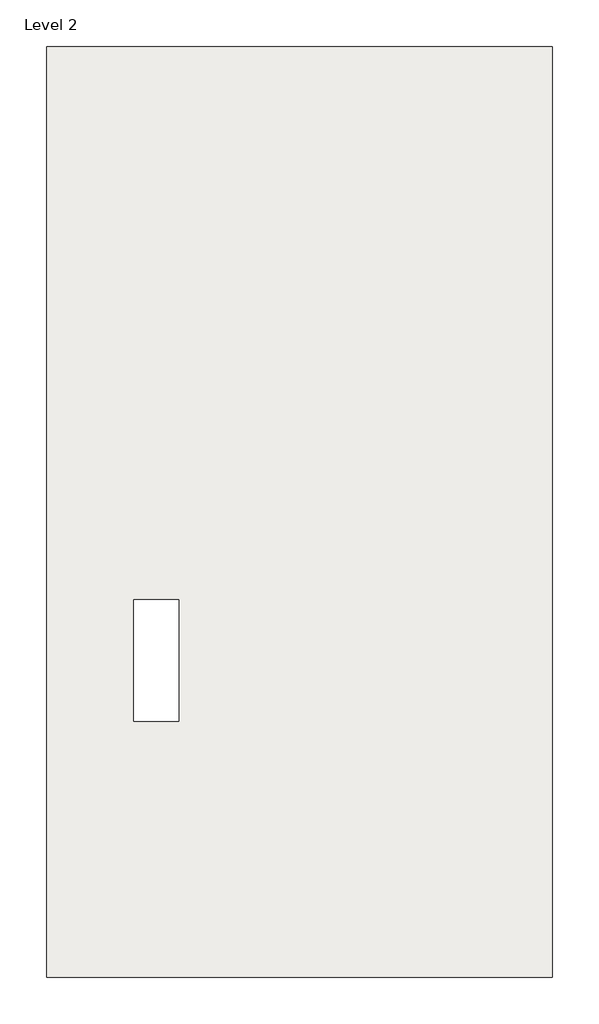
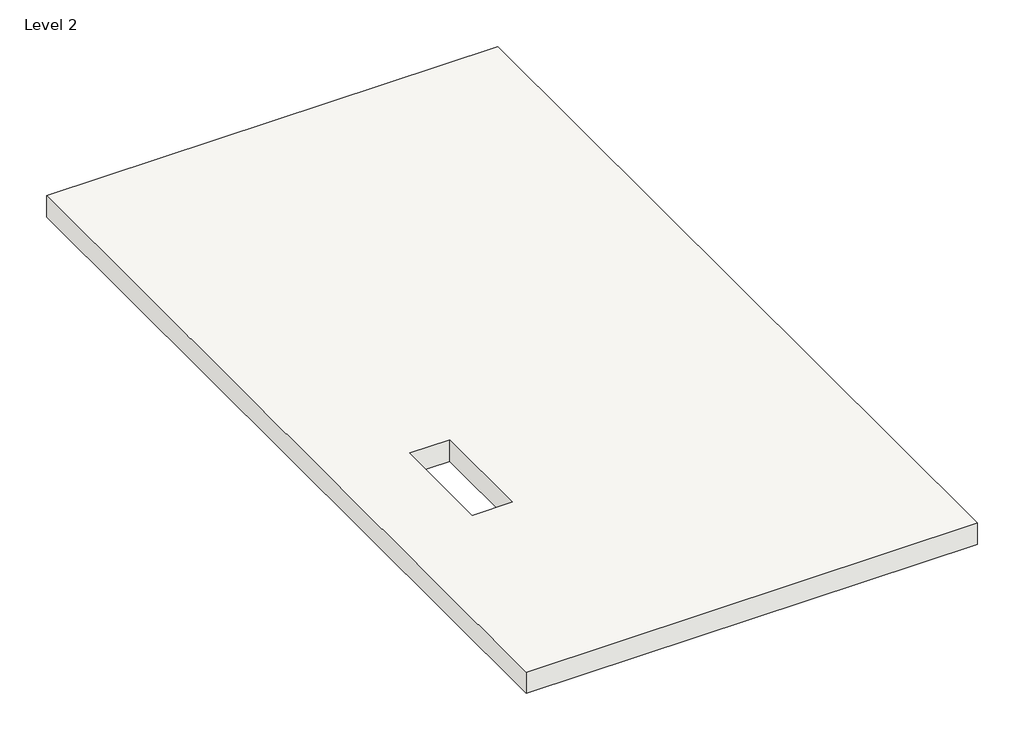
# One storey: 1 roof.
"""IFC4 building model written with IfcOpenShell, lengths in millimetres."""

from ifc_helpers import new_model, si_unit, frame, origin, place, context, project, spatial, polyline, outline, extrude, element, save

model = new_model("IFC4")

# Units and contexts
model_context = context("Model", 3, world=origin())
ifc_project = project(units=[si_unit("LENGTHUNIT", "METRE", prefix="MILLI")], contexts=[model_context])

# Site, building, storey
site = spatial("IfcSite", under=ifc_project)
building = spatial("IfcBuilding", under=site)
storey = spatial("IfcBuildingStorey", under=building, Name="Level 2", Elevation=3048.0)

# Roof
placement = place(None, origin())
element("IfcRoof", 1, ObjectType="Steel Truss - Insulation on Metal Deck - EPDM", at=placement, inside=storey, context=model_context, shape_type="SweptSolid", body=[
    extrude(outline(polyline([(-12479.1602428, 16732.1316988), (-1607.9602428, 16732.1316988), (-1607.9602428, -3283.0683012), (-12479.1602428, -3283.0683012), (-12479.1602428, 16732.1316988)]), holes=[polyline([(-10599.5602428, 4836.5398463), (-10599.5602428, 2220.3398463), (-9634.3602428, 2220.3398463), (-9634.3602428, 4836.5398463), (-10599.5602428, 4836.5398463)])]), frame((0.0, 0.0, 3048.0), z_axis=(0.0, 0.0, 1.0), x_axis=(1.0, 0.0, 0.0)), (0.0, 0.0, 1.0), 546.1),
])

save(model, "model.ifc")

# Revit data of these elements
# Type "Steel Truss - Insulation on Metal Deck - EPDM"
#   Assembly Code = "B1020"
#   Layers, outside or top first: 0' - 0 1/4" "Roofing, EPDM Membrane" (function 4); 0' - 5" "Rigid insulation" (function 3); 0' - 0 1/4" "Metal Deck" (function 1); 1' - 4" "Structure, Steel Bar Joist Layer" (function 1)
# Element 1 (IfcRoof, "Steel Truss - Insulation on Metal Deck - EPDM")
#   built-in parameter 1001705 = 11.7917 (stored number, unit not read)
#   built-in parameter 1001710 = 33615
#   Phase Created = New Construction
#   Materials on its faces: "Structure, Steel Bar Joist Layer", "Roofing, EPDM Membrane"
# Materials
#   "Roofing, EPDM Membrane": class "Generic", colour RGB 127 127 127, transparency 0, Description = "EPDM roof membrane", Cost = 0
#   "Rigid insulation": class "Generic", colour RGB 127 127 127, transparency 0, Description = "Rigid foam insulation board", Cost = 0
#   "Metal Deck": class "Metal", colour RGB 199 199 199, transparency 0, Description = "Steel, mill finish", Cost = 0
#   "Structure, Steel Bar Joist Layer": class "Metal", colour RGB 127 127 127, transparency 0, Description = "Bar joists, thermal airspace", Cost = 0
